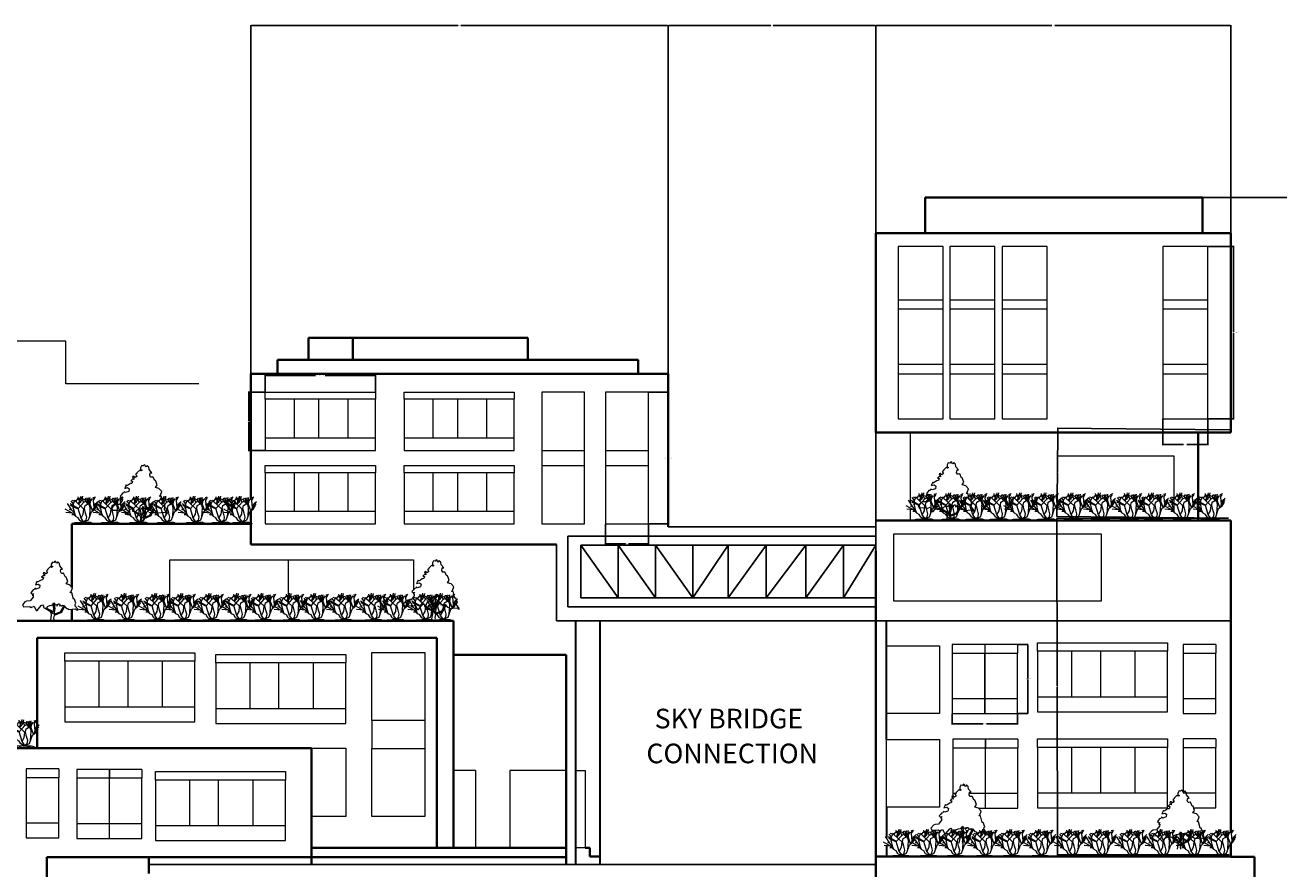
# Model space of a CAD drawing. Units: inches. Extents: x -934 to 898, y -1502 to 444.
# Tile 9 of 10: x -117 to 286, y -87 to 185. Entities that reach past the tile are written whole.
import ezdxf

# ---------------------------------------------------------------- set-up
doc = ezdxf.new("R2010")
doc.units = ezdxf.units.IN
doc.header["$MEASUREMENT"] = 0
for name, color, linetype, lineweight in [('A-ANNO-DIMS', 2, 'Continuous', 18), ('A-ANNO-TEXT', 7, 'Continuous', 18), ('A-COLS', 1, 'Continuous', 30), ('A-ELEV', 7, 'Continuous', 35), ('A-GLAZ', 4, 'Continuous', 13), ('A-ROOF', 7, 'Continuous', 35), ('L-PLNT-TREE', 3, 'Continuous', 13), ('S-BRDG', 5, 'Continuous', 25)]:
    doc.layers.add(name, color=color, linetype=linetype, lineweight=lineweight)
doc.styles.get("Standard").update_dxf_attribs({"font": 'arial.ttf'})
doc.dimstyles.get("Standard").update_dxf_attribs({"dimtxt": 0.18, "dimasz": 0.18, "dimexe": 0.18, "dimexo": 0.0625, "dimgap": 0.09, "dimtad": 0, "dimtih": 1, "dimtoh": 1, "dimdec": 4, "dimzin": 0, "dimdsep": 46, "dimtxsty": 'Standard', "dimcen": 0.09, "dimadec": 0, "dimazin": 0, "dimtfac": 1, "dimtdec": 4, "dimtofl": 0, "dimtmove": 0, "dimatfit": 3, "dimfxl": 1, "dimtolj": 1, "dimtzin": 0, "dimarcsym": 0})

# ---------------------------------------------------------------- blocks, each defined once
blk = doc.blocks.new('*U2')
for points in [[(22.0124, 137.721), (18.5475, 141.5624), (15.5282, 138.2446), (13.8028, 139.3505), (13.3714, 142.1153), (11.2148, 143.2214), (8.1954, 140.4564), (4.7447, 141.0094), (2.1567, 136.0326), (2.1567, 131.6088), (5.6074, 129.9499), (3.0193, 128.2909), (0.4313, 130.5029), (-6.9015, 123.3141), (-6.9015, 121.6552), (-9.9208, 119.9963), (-9.0581, 118.3373), (-6.9015, 115.0195), (-10.7835, 112.2546), (-14.6656, 115.0195), (-16.8222, 114.4665), (-17.6849, 112.2546), (-14.6656, 111.7016), (-14.2342, 107.2778), (-17.6065, 107.8307), (-21.5669, 103.9599), (-17.2536, 103.4069), (-18.9789, 97.8771), (-22.8609, 97.3241), (-27.1743, 94.5593), (-32.3504, 91.7944), (-32.7817, 94.0063), (-36.6638, 85.7116), (-29.7624, 87.3705), (-25.449, 84.6056), (-26.743, 77.9699), (-34.507, 75.205), (-37.9578, 77.4169), (-39.2518, 74.099), (-42.2711, 73.5461), (-44.8592, 70.2282), (-47.8786, 66.3574), (-43.9965, 63.0395), (-41.4085, 64.6985), (-44.3346, 59.8898), (-42.2089, 60.1377), (-42.5159, 55.7849), (-49.6039, 46.4502), (-58.2307, 45.8972), (-62.1127, 43.6853), (-68.5828, 36.4966), (-65.9947, 32.0727), (-50.0352, 32.6257), (-47.0159, 30.4138), (-39.6831, 33.7317), (-34.507, 22.6721), (-32.3504, 22.6721), (-22.4296, 34.8376), (-19.4102, 36.4966), (-17.2536, 33.7317), (-17.2536, 29.8608), (-13.8028, 28.7549), (-9.0581, 28.7549), (-7.3328, 32.6257), (-1.7254, 35.3906), (3.8821, 35.9436), (6.4701, 38.1555), (6.9014, 38.7085), (8.1954, 41.4734), (9.9208, 40.3674), (11.2148, 35.9436), (14.2341, 37.6025), (15.0968, 36.4966), (15.9595, 33.7317), (18.9789, 38.7085), (21.9982, 38.7085), (23.2922, 36.4966), (21.9982, 34.2847), (25.4489, 35.3906), (26.743, 33.7317), (29.7623, 35.9436), (32.7817, 34.8376), (38.8204, 28.7549), (41.4084, 27.6489), (43.5651, 25.437), (61.6813, 27.0959), (65.132, 23.7781), (67.7201, 24.884), (60.8186, 33.7317), (60.3873, 37.0495), (62.544, 40.3674), (58.662, 50.874), (56.5053, 50.874), (52.1919, 66.3574), (47.8785, 66.9103), (50.4665, 69.1222), (53.9172, 77.9699), (47.0158, 85.1586), (38.3891, 87.9235), (42.2711, 94.0063)], [(42.2711, 94.0063), (38.8204, 104.5129), (36.6637, 104.5129), (32.3503, 113.9135), (29.7623, 113.3605), (26.743, 113.3605), (24.5862, 117.7844), (25.8802, 123.8671), (29.331, 123.8671), (22.8609, 131.6088), (21.9982, 137.6916)], [(-9.9208, 28.2019), (0, 23.2251), (3.4507, 19.9072), (4.7447, 15.4834), (8.6267, 27.0959), (6.4701, 37.6025)], [(34.5071, 33.1787), (27.1743, 18.2483), (9.0581, 10.5066), (7.7641, 3.8708), (8.1954, 0)], [(8.1954, 40.3674), (11.2148, 27.6489), (8.1954, 13.8245), (24.5862, 19.9072), (32.7817, 34.2847)], [(-12.9401, 28.7549), (-2.588, 22.1191), (0.8626, 17.6953), (1.7253, 11.6125), (0, 0)]]:
    blk.add_lwpolyline(points)
blk = doc.blocks.new('*U6')
for p, q in [((-316.7634, 502.285), (-327.6092, 559.9176)), ((-286.512, 498.3226), (-307.4416, 538.0736)), ((-290.3982, 464.5406), (-265.6078, 577.8246)), ((-207.264, 451.104), (-268.224, 548.64)), ((-240.792, 502.285), (-228.3968, 573.8368)), ((-182.88, 499.872), (-158.496, 536.448)), ((-129.1844, 450.6214), (-140.0302, 542.036)), ((-134.112, 487.68), (-97.536, 548.64)), ((-85.7758, 472.4908), (-73.3552, 548.005)), ((-12.9032, 555.9552), (-2.0574, 522.1732)), ((-5.1562, 486.3846), (2.5908, 542.036)), ((-0.508, 508.254), (22.7584, 536.067)), ((1.0414, 526.1356), (35.1536, 559.9176)), ((2.5908, 542.036), (21.209, 555.9552)), ((-451.104, 219.456), (-601.0402, 303.8094)), ((-463.296, 280.416), (-552.577, 423.037)), ((-463.296, 280.416), (-512.064, 292.608)), ((-329.184, 316.992), (-499.872, 414.528)), ((-353.568, 316.992), (-487.68, 377.952)), ((-426.72, 414.528), (-475.488, 475.488)), ((-402.336, 207.264), (-463.296, 280.416)), ((-377.952, 463.296), (-451.104, 487.68)), ((-426.72, 316.992), (-451.104, 329.184)), ((-426.72, 414.528), (-390.144, 499.872)), ((-426.72, 316.992), (-426.72, 414.528)), ((-402.336, 207.264), (-426.72, 316.992)), ((-377.952, 463.296), (-329.184, 524.256)), ((-207.264, 304.8), (-377.952, 463.296)), ((-329.184, 316.992), (-353.568, 316.992)), ((-338.455, 424.7896), (-290.3982, 464.5406)), ((-329.184, 316.992), (-207.264, 451.104)), ((-268.224, 109.728), (-329.184, 316.992)), ((-296.5958, 484.4034), (-316.7634, 502.285)), ((-305.8922, 396.9512), (-302.7934, 478.4344)), ((-304.3428, 426.7708), (-268.7066, 458.5716)), ((-302.7934, 478.4344), (-270.256, 518.1854)), ((-268.7066, 458.5716), (-250.0884, 500.3038)), ((-182.88, 499.872), (-219.456, 512.064)), ((-219.456, 195.072), (-207.264, 304.8)), ((-207.264, 451.104), (-134.112, 487.68)), ((-195.072, 316.992), (-182.88, 377.952)), ((-170.688, 219.456), (-195.072, 316.992)), ((-121.92, 414.528), (-182.88, 499.872)), ((-182.88, 377.952), (-97.536, 426.72)), ((-85.7758, 389.001), (-129.1844, 452.6026)), ((-73.152, 329.184), (-109.728, 499.872)), ((-97.536, 426.72), (-24.384, 524.256)), ((-70.2564, 426.7708), (-85.7758, 472.4908)), ((-85.344, 134.112), (-73.152, 329.184)), ((-73.152, 402.336), (-60.96, 512.064)), ((-24.384, 268.224), (-73.152, 402.336)), ((-48.768, 243.84), (24.384, 304.8)), ((-12.192, 274.32), (8.7884, 335.3562)), ((8.7884, 335.3562), (-5.1562, 486.3846)), ((-3.6068, 492.3536), (14.986, 518.1854)), ((8.7884, 335.3562), (33.6042, 412.8516)), ((24.384, 304.8), (36.576, 390.144)), ((24.384, 304.8), (73.152, 377.952)), ((33.6042, 412.8516), (92.5068, 464.5406)), ((36.576, 390.144), (73.152, 438.912)), ((48.768, 341.376), (60.96, 390.144)), ((60.96, 390.144), (85.344, 414.528)), ((-451.104, 219.456), (-587.4512, 234.2388)), ((-414.528, 182.88), (-463.296, 182.88)), ((-377.952, 146.304), (-451.104, 219.456)), ((-402.336, 12.192), (-451.104, 0)), ((-377.952, 146.304), (-402.336, 207.264)), ((-341.376, 12.192), (-402.336, 12.192)), ((-329.184, 121.92), (-377.952, 146.304)), ((-243.84, 24.384), (-341.376, 12.192)), ((-292.608, 60.96), (-329.184, 121.92)), ((-243.84, 24.384), (-329.184, 0)), ((-219.456, 24.384), (-292.608, 60.96)), ((-268.224, 109.728), (-219.456, 195.072)), ((-219.456, 48.768), (-268.224, 109.728)), ((-243.84, 24.384), (-195.072, 24.384)), ((-219.456, 24.384), (-109.728, 73.152)), ((-219.456, 24.384), (-158.496, 73.152)), ((-219.456, 24.384), (-219.456, 48.768)), ((-219.456, 24.384), (-73.152, 24.384)), ((-195.072, 24.384), (-158.496, 12.192)), ((-146.304, 134.112), (-170.688, 219.456)), ((-158.496, 73.152), (-146.304, 134.112)), ((-158.496, 12.192), (-85.344, 0)), ((-109.728, 73.152), (-48.768, 243.84)), ((-73.152, 24.384), (0, 0))]:
    blk.add_line(p, q)
blk = doc.blocks.new('*U4')
for points in [[(559.11496, 3498.1134), (471.1065, 3595.68496), (394.41628, 3511.41284), (350.59112, 3539.5027), (339.63356, 3609.72862), (284.85592, 3637.82356), (208.16316, 3567.59256), (120.51538, 3581.63876), (54.78018, 3455.22804), (54.78018, 3342.86352), (142.42796, 3300.72746), (76.69022, 3258.58886), (10.95502, 3314.77366), (-175.2981, 3132.17814), (-175.2981, 3090.04208), (-251.98832, 3047.90602), (-230.07574, 3005.76742), (-175.2981, 2921.4953), (-273.9009, 2851.26684), (-372.50624, 2921.4953), (-427.28388, 2907.4491), (-449.19646, 2851.26684), (-372.50624, 2837.22064), (-361.54868, 2724.85612), (-447.2051, 2738.89978), (-547.79926, 2640.58146), (-438.24144, 2626.53526), (-482.06406, 2486.07834), (-580.66686, 2472.03214), (-690.22722, 2401.80622), (-821.70016, 2331.57776), (-832.65518, 2387.76002), (-931.26052, 2177.07464), (-755.96496, 2219.2107), (-646.4046, 2148.98224), (-679.2722, 1980.43546), (-876.4778, 1910.207), (-964.12812, 1966.38926), (-996.99572, 1882.1146), (-1073.68594, 1868.07094), (-1139.42368, 1783.79628), (-1216.11644, 1685.47796), (-1117.5111, 1601.2033), (-1051.7759, 1643.3419), (-1126.09884, 1521.20092), (-1072.10606, 1527.49758), (-1079.90386, 1416.93646), (-1259.93906, 1179.83508), (-1479.05978, 1165.78888), (-1577.66258, 1109.60662), (-1742.00312, 927.01364), (-1676.26538, 814.64658), (-1270.89408, 828.69278), (-1194.20386, 772.51052), (-1007.95074, 856.78518), (-876.4778, 575.87134), (-821.70016, 575.87134), (-569.71184, 884.87504), (-493.01908, 927.01364), (-438.24144, 856.78518), (-438.24144, 758.46432), (-350.59112, 730.37446), (-230.07574, 730.37446), (-186.25312, 828.69278), (-43.82516, 898.92124), (98.60534, 912.96744), (164.34054, 969.1497), (175.29556, 983.1959), (208.16316, 1053.42436), (251.98832, 1025.33196), (284.85592, 912.96744), (361.54614, 955.1035), (383.45872, 927.01364), (405.3713, 856.78518), (482.06406, 983.1959), (558.75428, 983.1959), (591.62188, 927.01364), (558.75428, 870.83138), (646.40206, 898.92124), (679.2722, 856.78518), (755.96242, 912.96744), (832.65518, 884.87504), (986.03816, 730.37446), (1051.77336, 702.28206), (1106.55354, 646.0998), (1566.70502, 688.23586), (1654.3528, 603.96374), (1720.09054, 632.0536), (1544.79244, 856.78518), (1533.83742, 941.0573), (1588.6176, 1025.33196), (1490.0148, 1292.1996), (1435.23462, 1292.1996), (1325.67426, 1685.47796), (1216.1139, 1699.52162), (1281.8491, 1755.70388), (1369.49688, 1980.43546), (1194.20132, 2163.02844), (975.08314, 2233.2569), (1073.68594, 2387.76002)], [(1073.68594, 2387.76002), (986.03816, 2654.62766), (931.25798, 2654.62766), (821.69762, 2893.4029), (755.96242, 2879.3567), (679.2722, 2879.3567), (624.48948, 2991.72376), (657.35708, 3146.22434), (745.0074, 3146.22434), (580.66686, 3342.86352), (558.75428, 3497.36664)], [(-251.98832, 716.32826), (0, 589.91754), (87.64778, 505.64288), (120.51538, 393.27836), (219.11818, 688.23586), (164.34054, 955.1035)], [(876.48034, 842.73898), (690.22722, 463.50682), (230.07574, 266.86764), (197.20814, 98.31832), (208.16316, 0)], [(208.16316, 1025.33196), (284.85592, 702.28206), (208.16316, 351.1423), (624.48948, 505.64288), (832.65518, 870.83138)], [(-328.67854, 730.37446), (-65.7352, 561.82514), (21.91004, 449.46062), (43.82262, 294.9575), (0, 0)]]:
    blk.add_lwpolyline(points)
blk = doc.blocks.new('WIN-TWIN-NARROW')
for p, q in [((10.5, 22.21), (0, 22.21)), ((0, 22.21), (0, 19.45)), ((20.91, 22.21), (10.41, 22.21)), ((10.41, 22.21), (10.41, 19.45)), ((10.5, 22.21), (10.5, 19.45)), ((20.91, 22.21), (20.91, 19.45)), ((0, 19.45), (0, 4.84)), ((0, 19.45), (10.5, 19.45)), ((10.41, 19.45), (10.41, 4.84)), ((10.41, 19.45), (20.91, 19.45)), ((10.5, 4.84), (10.5, 19.45)), ((20.91, 4.84), (20.91, 19.45)), ((0, 4.84), (10.5, 4.84)), ((0, 4.84), (0, 0)), ((10.41, 4.84), (20.91, 4.84)), ((10.41, 4.84), (10.41, 0)), ((10.5, 0), (10.5, 4.84)), ((20.91, 0), (20.91, 4.84)), ((0, 0), (10.5, 0)), ((10.41, 0), (20.91, 0))]:
    blk.add_line(p, q)
blk = doc.blocks.new('WIN-SINGLE-NARROW')
for p, q in [((10.5, 22.21), (0, 22.21)), ((0, 22.21), (0, 19.45)), ((10.5, 22.21), (10.5, 19.45)), ((0, 19.45), (0, 4.84)), ((0, 19.45), (10.5, 19.45)), ((10.5, 4.84), (10.5, 19.45)), ((0, 4.84), (10.5, 4.84)), ((0, 4.84), (0, 0)), ((10.5, 0), (10.5, 4.84)), ((0, 0), (10.5, 0))]:
    blk.add_line(p, q)
blk = doc.blocks.new('WIN-RIBBON-LARGE')
for p, q in [((0, 19.45), (0, 22.21)), ((0, 22.21), (41.85, 22.21)), ((41.85, 22.21), (41.85, 19.45)), ((0, 19.45), (0, 4.84)), ((41.85, 19.45), (0, 19.45)), ((10.96, 19.45), (10.96, 4.84)), ((20.23, 19.45), (20.23, 4.84)), ((31.34, 19.45), (31.34, 4.84)), ((41.85, 4.84), (41.85, 19.45)), ((0, 4.84), (41.85, 4.84)), ((0, 4.84), (0, 0)), ((41.85, 0), (41.85, 4.84)), ((0, 0), (41.85, 0))]:
    blk.add_line(p, q)
blk = doc.blocks.new('WIN-RIBBON-COMPACT')
for p, q in [((0, 16.47), (0, 18.8)), ((0, 18.8), (35.42, 18.8)), ((0, 16.47), (0, 4.09)), ((35.42, 16.47), (0, 16.47)), ((9.28, 16.47), (9.28, 4.09)), ((17.13, 16.47), (17.13, 4.09)), ((26.53, 16.47), (26.53, 4.09)), ((35.42, 18.8), (35.42, 16.47)), ((35.42, 4.09), (35.42, 16.47)), ((0, 4.09), (35.42, 4.09)), ((0, 4.09), (0, 0)), ((35.42, 0), (35.42, 4.09)), ((0, 0), (35.42, 0))]:
    blk.add_line(p, q)
blk = doc.blocks.new('WIN-TOWER-STACK')
for p, q in [((0, 55.38), (0, 0)), ((14.46, 55.38), (0, 55.38)), ((14.46, 0), (14.46, 55.38)), ((0, 38.19), (14.46, 38.19)), ((0, 35.32), (14.46, 35.32)), ((0, 17.59), (14.46, 17.59)), ((0, 14.39), (14.46, 14.39)), ((0, 0), (14.46, 0))]:
    blk.add_line(p, q)
blk = doc.blocks.new('WIN-VERTICAL-LIGHT')
for p, q in [((0, 42.42), (0, 0)), ((13.76, 42.42), (0, 42.42)), ((13.76, 0), (13.76, 42.42)), ((0, 23.62), (13.76, 23.62)), ((0, 18.8), (13.76, 18.8)), ((0, 0), (13.76, 0))]:
    blk.add_line(p, q)
blk = doc.blocks.new('*D35')
at = {"layer": 'A-ANNO-DIMS', "color": 0, "lineweight": -2, "transparency": 16777216}
for p, q in [((202.02, -14.7), (205.47, -14.7)), ((205.29, -14.88), (205.29, -25.62)), ((205.29, -36.73), (205.29, -25.99)), ((202.02, -36.91), (205.47, -36.91))]:
    blk.add_line(p, q, dxfattribs=at)
at = {"layer": 'A-ANNO-DIMS', "color": 0, "transparency": 16777216}
for points in [[(205.26, -14.88), (205.32, -14.88), (205.29, -14.7)], [(205.26, -36.73), (205.32, -36.73), (205.29, -36.91)]]:
    blk.add_solid(points, dxfattribs=at)
at = {"layer": 'Defpoints', "color": 0, "transparency": 16777216}
for p in [(201.96, -14.7), (205.29, -14.7), (201.96, -36.91)]:
    blk.add_point(p, dxfattribs=at)
at = {"layer": 'A-ANNO-DIMS', "color": 0, "transparency": 16777216, "insert": (205.29, -25.8), "char_height": 0.18, "attachment_point": 5}
blk.add_mtext('\\A1;SLIM TWIN 22 TYP.', dxfattribs=at)
blk = doc.blocks.new('*D36')
at = {"layer": 'A-ANNO-DIMS', "color": 0, "lineweight": -2, "transparency": 16777216}
for p, q in [((181.05, -36.97), (181.05, -40.42)), ((181.23, -40.24), (190.98, -40.24)), ((201.78, -40.24), (192.04, -40.24)), ((201.96, -36.97), (201.96, -40.42))]:
    blk.add_line(p, q, dxfattribs=at)
at = {"layer": 'A-ANNO-DIMS', "color": 0, "transparency": 16777216}
for points in [[(181.23, -40.21), (181.23, -40.27), (181.05, -40.24)], [(201.78, -40.21), (201.78, -40.27), (201.96, -40.24)]]:
    blk.add_solid(points, dxfattribs=at)
at = {"layer": 'Defpoints', "color": 0, "transparency": 16777216}
for p in [(181.05, -36.91), (201.96, -36.91), (201.96, -40.24)]:
    blk.add_point(p, dxfattribs=at)
at = {"layer": 'A-ANNO-DIMS', "color": 0, "transparency": 16777216, "insert": (191.51, -40.24), "char_height": 0.18, "attachment_point": 5}
blk.add_mtext('\\A1;21 TYP.', dxfattribs=at)
blk = doc.blocks.new('*D41')
at = {"layer": 'A-ANNO-DIMS', "color": 0, "lineweight": -2, "transparency": 16777216}
for p, q in [((-39.96, 66.58), (-39.96, 72.01)), ((-39.78, 71.83), (-23.77, 71.83)), ((-4.72, 71.83), (-20.73, 71.83)), ((-4.54, 66.58), (-4.54, 72.01))]:
    blk.add_line(p, q, dxfattribs=at)
at = {"layer": 'A-ANNO-DIMS', "color": 0, "transparency": 16777216}
for points in [[(-39.78, 71.86), (-39.78, 71.8), (-39.96, 71.83)], [(-4.72, 71.86), (-4.72, 71.8), (-4.54, 71.83)]]:
    blk.add_solid(points, dxfattribs=at)
at = {"layer": 'Defpoints', "color": 0, "transparency": 16777216}
for p in [(-4.54, 71.83), (-39.96, 66.52), (-4.54, 66.52)]:
    blk.add_point(p, dxfattribs=at)
at = {"layer": 'A-ANNO-DIMS', "color": 0, "transparency": 16777216, "insert": (-22.25, 71.83), "char_height": 0.18, "attachment_point": 5}
blk.add_mtext('\\A1;SHORT RIBBON 35 TYP.', dxfattribs=at)
blk = doc.blocks.new('*D42')
at = {"layer": 'A-ANNO-DIMS', "color": 0, "lineweight": -2, "transparency": 16777216}
for p, q in [((-40.03, 66.52), (-45.46, 66.52)), ((-45.28, 66.34), (-45.28, 57.3)), ((-45.28, 47.9), (-45.28, 56.94)), ((-40.03, 47.72), (-45.46, 47.72))]:
    blk.add_line(p, q, dxfattribs=at)
at = {"layer": 'A-ANNO-DIMS', "color": 0, "transparency": 16777216}
for points in [[(-45.31, 66.34), (-45.25, 66.34), (-45.28, 66.52)], [(-45.31, 47.9), (-45.25, 47.9), (-45.28, 47.72)]]:
    blk.add_solid(points, dxfattribs=at)
at = {"layer": 'Defpoints', "color": 0, "transparency": 16777216}
for p in [(-45.28, 66.52), (-39.96, 66.52), (-39.96, 47.72)]:
    blk.add_point(p, dxfattribs=at)
at = {"layer": 'A-ANNO-DIMS', "color": 0, "transparency": 16777216, "insert": (-45.28, 57.12), "char_height": 0.18, "attachment_point": 5}
blk.add_mtext('\\A1;19 TYP.', dxfattribs=at)
blk = doc.blocks.new('*D43')
at = {"layer": 'A-ANNO-DIMS', "color": 0, "lineweight": -2, "transparency": 16777216}
for p, q in [((263.27, 113.31), (271.69, 113.31)), ((271.51, 113.13), (271.51, 85.81)), ((271.51, 58.11), (271.51, 85.44)), ((263.27, 57.93), (271.69, 57.93))]:
    blk.add_line(p, q, dxfattribs=at)
at = {"layer": 'A-ANNO-DIMS', "color": 0, "transparency": 16777216}
for points in [[(271.48, 113.13), (271.54, 113.13), (271.51, 113.31)], [(271.48, 58.11), (271.54, 58.11), (271.51, 57.93)]]:
    blk.add_solid(points, dxfattribs=at)
at = {"layer": 'Defpoints', "color": 0, "transparency": 16777216}
for p in [(263.21, 113.31), (271.51, 113.31), (263.21, 57.93)]:
    blk.add_point(p, dxfattribs=at)
at = {"layer": 'A-ANNO-DIMS', "color": 0, "transparency": 16777216, "insert": (271.51, 85.62), "char_height": 0.18, "attachment_point": 5}
blk.add_mtext('\\A1;TOWER LIGHT 55 TYP.', dxfattribs=at)
blk = doc.blocks.new('*D44')
at = {"layer": 'A-ANNO-DIMS', "color": 0, "lineweight": -2, "transparency": 16777216}
for p, q in [((248.75, 57.87), (248.75, 49.45)), ((263.21, 57.87), (263.21, 49.45)), ((248.93, 49.63), (255.46, 49.63)), ((263.03, 49.63), (256.5, 49.63))]:
    blk.add_line(p, q, dxfattribs=at)
at = {"layer": 'A-ANNO-DIMS', "color": 0, "transparency": 16777216}
for points in [[(248.93, 49.66), (248.93, 49.6), (248.75, 49.63)], [(263.03, 49.66), (263.03, 49.6), (263.21, 49.63)]]:
    blk.add_solid(points, dxfattribs=at)
at = {"layer": 'Defpoints', "color": 0, "transparency": 16777216}
for p in [(248.75, 57.93), (263.21, 57.93), (263.21, 49.63)]:
    blk.add_point(p, dxfattribs=at)
at = {"layer": 'A-ANNO-DIMS', "color": 0, "transparency": 16777216, "insert": (255.98, 49.63), "char_height": 0.18, "attachment_point": 5}
blk.add_mtext('\\A1;14 TYP.', dxfattribs=at)
blk = doc.blocks.new('*D45')
at = {"layer": 'A-ANNO-DIMS', "color": 0, "lineweight": -2, "transparency": 16777216}
for p, q in [((83.35, 66.52), (89.83, 66.52)), ((89.65, 66.34), (89.65, 45.49)), ((89.65, 24.28), (89.65, 45.12)), ((83.35, 24.1), (89.83, 24.1))]:
    blk.add_line(p, q, dxfattribs=at)
at = {"layer": 'A-ANNO-DIMS', "color": 0, "transparency": 16777216}
for points in [[(89.62, 66.34), (89.68, 66.34), (89.65, 66.52)], [(89.62, 24.28), (89.68, 24.28), (89.65, 24.1)]]:
    blk.add_solid(points, dxfattribs=at)
at = {"layer": 'Defpoints', "color": 0, "transparency": 16777216}
for p in [(83.29, 66.52), (89.65, 66.52), (83.29, 24.1)]:
    blk.add_point(p, dxfattribs=at)
at = {"layer": 'A-ANNO-DIMS', "color": 0, "transparency": 16777216, "insert": (89.65, 45.31), "char_height": 0.18, "attachment_point": 5}
blk.add_mtext('\\A1;VERT. LIGHT 42 TYP.', dxfattribs=at)
blk = doc.blocks.new('*D46')
at = {"layer": 'A-ANNO-DIMS', "color": 0, "lineweight": -2, "transparency": 16777216}
for p, q in [((69.53, 24.03), (69.53, 17.55)), ((83.29, 24.03), (83.29, 17.55)), ((69.71, 17.73), (75.89, 17.73)), ((83.11, 17.73), (76.93, 17.73))]:
    blk.add_line(p, q, dxfattribs=at)
at = {"layer": 'A-ANNO-DIMS', "color": 0, "transparency": 16777216}
for points in [[(69.71, 17.76), (69.71, 17.7), (69.53, 17.73)], [(83.11, 17.76), (83.11, 17.7), (83.29, 17.73)]]:
    blk.add_solid(points, dxfattribs=at)
at = {"layer": 'Defpoints', "color": 0, "transparency": 16777216}
for p in [(69.53, 24.1), (83.29, 24.1), (83.29, 17.73)]:
    blk.add_point(p, dxfattribs=at)
at = {"layer": 'A-ANNO-DIMS', "color": 0, "transparency": 16777216, "insert": (76.41, 17.73), "char_height": 0.18, "attachment_point": 5}
blk.add_mtext('\\A1;14 TYP.', dxfattribs=at)
blk = doc.blocks.new('*D80')
at = {"layer": 'A-ANNO-DIMS', "color": 0, "lineweight": -2, "transparency": 16777216}
for p, q in [((261.62, 129.1), (464.31, 129.1)), ((464.13, 128.92), (464.13, -24.61)), ((464.13, -178.5), (464.13, -24.97)), ((239.7, -178.68), (464.31, -178.68))]:
    blk.add_line(p, q, dxfattribs=at)
at = {"layer": 'A-ANNO-DIMS', "color": 0, "transparency": 16777216}
for points in [[(464.1, 128.92), (464.16, 128.92), (464.13, 129.1)], [(464.1, -178.5), (464.16, -178.5), (464.13, -178.68)]]:
    blk.add_solid(points, dxfattribs=at)
at = {"layer": 'Defpoints', "color": 0, "transparency": 16777216}
for p in [(261.56, 129.1), (464.13, 129.1), (239.64, -178.68)]:
    blk.add_point(p, dxfattribs=at)
at = {"layer": 'A-ANNO-DIMS', "color": 0, "transparency": 16777216, "insert": (464.13, -24.79), "char_height": 0.18, "attachment_point": 5}
blk.add_mtext('\\A1;307.8', dxfattribs=at)
blk = doc.blocks.new('*D83')
at = {"layer": 'A-ANNO-DIMS', "color": 0, "lineweight": -2, "transparency": 16777216}
for p, q in [((156.42, 117.65), (156.42, 184.53)), ((156.6, 184.35), (213.08, 184.35)), ((270.46, 184.35), (213.99, 184.35)), ((270.64, 117.65), (270.64, 184.53))]:
    blk.add_line(p, q, dxfattribs=at)
at = {"layer": 'A-ANNO-DIMS', "color": 0, "transparency": 16777216}
for points in [[(156.6, 184.38), (156.6, 184.32), (156.42, 184.35)], [(270.46, 184.38), (270.46, 184.32), (270.64, 184.35)]]:
    blk.add_solid(points, dxfattribs=at)
at = {"layer": 'Defpoints', "color": 0, "transparency": 16777216}
for p in [(270.64, 184.35), (156.42, 117.59), (270.64, 117.59)]:
    blk.add_point(p, dxfattribs=at)
at = {"layer": 'A-ANNO-DIMS', "color": 0, "transparency": 16777216, "insert": (213.53, 184.35), "char_height": 0.18, "attachment_point": 5}
blk.add_mtext('\\A1;114.22', dxfattribs=at)
blk = doc.blocks.new('*D86')
at = {"layer": 'A-ANNO-DIMS', "color": 0, "lineweight": -2, "transparency": 16777216}
for p, q in [((-44.58, 72.4), (-44.58, 184.53)), ((-44.4, 184.35), (22.08, 184.35)), ((89.46, 184.35), (22.98, 184.35)), ((89.64, 72.4), (89.64, 184.53))]:
    blk.add_line(p, q, dxfattribs=at)
at = {"layer": 'A-ANNO-DIMS', "color": 0, "transparency": 16777216}
for points in [[(-44.4, 184.38), (-44.4, 184.32), (-44.58, 184.35)], [(89.46, 184.38), (89.46, 184.32), (89.64, 184.35)]]:
    blk.add_solid(points, dxfattribs=at)
at = {"layer": 'Defpoints', "color": 0, "transparency": 16777216}
for p in [(89.64, 184.35), (-44.58, 72.34), (89.64, 72.34)]:
    blk.add_point(p, dxfattribs=at)
at = {"layer": 'A-ANNO-DIMS', "color": 0, "transparency": 16777216, "insert": (22.53, 184.35), "char_height": 0.18, "attachment_point": 5}
blk.add_mtext('\\A1;134.22', dxfattribs=at)
blk = doc.blocks.new('*D87')
at = {"layer": 'A-ANNO-DIMS', "color": 0, "lineweight": -2, "transparency": 16777216}
for p, q in [((89.64, 23.19), (89.64, 184.53)), ((89.82, 184.35), (122.64, 184.35)), ((156.24, 184.35), (123.43, 184.35)), ((156.42, 23.19), (156.42, 184.53))]:
    blk.add_line(p, q, dxfattribs=at)
at = {"layer": 'A-ANNO-DIMS', "color": 0, "transparency": 16777216}
for points in [[(89.82, 184.38), (89.82, 184.32), (89.64, 184.35)], [(156.24, 184.38), (156.24, 184.32), (156.42, 184.35)]]:
    blk.add_solid(points, dxfattribs=at)
at = {"layer": 'Defpoints', "color": 0, "transparency": 16777216}
for p in [(156.42, 184.35), (89.64, 23.13), (156.42, 23.13)]:
    blk.add_point(p, dxfattribs=at)
at = {"layer": 'A-ANNO-DIMS', "color": 0, "transparency": 16777216, "insert": (123.03, 184.35), "char_height": 0.18, "attachment_point": 5}
blk.add_mtext('\\A1;66.78', dxfattribs=at)
blk = doc.blocks.new('*D89')
at = {"layer": 'A-ANNO-DIMS', "color": 0, "lineweight": -2, "transparency": 16777216}
for p, q in [((270.16, 54.39), (214.8, 54.91)), ((214.98, 54.73), (214.85, 40.87)), ((214.71, 26.64), (214.84, 40.5)), ((269.89, 25.94), (214.53, 26.46))]:
    blk.add_line(p, q, dxfattribs=at)
at = {"layer": 'A-ANNO-DIMS', "color": 0, "transparency": 16777216}
for points in [[(214.95, 54.73), (215.01, 54.73), (214.98, 54.91)], [(214.68, 26.64), (214.74, 26.64), (214.71, 26.46)]]:
    blk.add_solid(points, dxfattribs=at)
at = {"layer": 'Defpoints', "color": 0, "transparency": 16777216}
for p in [(214.98, 54.91), (270.23, 54.39), (269.96, 25.94)]:
    blk.add_point(p, dxfattribs=at)
at = {"layer": 'A-ANNO-DIMS', "color": 0, "transparency": 16777216, "insert": (214.84, 40.69), "char_height": 0.18, "attachment_point": 5}
blk.add_mtext('\\A1;28.45', dxfattribs=at)
blk = doc.blocks.new('*D90')
at = {"layer": 'A-ANNO-DIMS', "color": 0, "lineweight": -2, "transparency": 16777216}
for p, q in [((269.89, 25.94), (214.53, 25.86)), ((214.71, 25.68), (214.78, -28.06)), ((214.86, -82.15), (214.78, -28.42)), ((270.05, -82.26), (214.68, -82.33))]:
    blk.add_line(p, q, dxfattribs=at)
at = {"layer": 'A-ANNO-DIMS', "color": 0, "transparency": 16777216}
for points in [[(214.74, 25.68), (214.68, 25.68), (214.71, 25.86)], [(214.89, -82.15), (214.83, -82.15), (214.86, -82.33)]]:
    blk.add_solid(points, dxfattribs=at)
at = {"layer": 'Defpoints', "color": 0, "transparency": 16777216}
for p in [(214.71, 25.86), (269.96, 25.94), (270.11, -82.26)]:
    blk.add_point(p, dxfattribs=at)
at = {"layer": 'A-ANNO-DIMS', "color": 0, "transparency": 16777216, "insert": (214.78, -28.24), "char_height": 0.18, "attachment_point": 5}
blk.add_mtext('\\A1;108.2', dxfattribs=at)

msp = doc.modelspace()

# ---------------------------------------------------------------- linework, layer by layer
at = {"layer": 'A-ANNO-TEXT'}
for p, q in [((-104.1148, 82.8773), (-138.836, 82.8773)), ((-104.1148, 69.1437), (-104.1148, 82.8773)), ((-61.3585, 69.1437), (-104.1148, 69.1437))]:
    msp.add_line(p, q, dxfattribs=at)
at = {"layer": 'A-COLS'}
for p, q in [((59.8691, -7.0768), (59.8691, -85.4234)), ((67.6239, -7.0768), (67.6239, -85.4234)), ((159.8346, -45.2684), (159.8346, -7.0768)), ((159.8346, -67.0531), (159.8346, -76.8096)), ((159.8346, -79.401), (159.8346, -82.9144))]:
    msp.add_line(p, q, dxfattribs=at)
at = {"layer": 'A-ELEV'}
for p, q in [((156.4222, 117.5909), (270.6435, 117.5909)), ((156.4222, 53.4791), (156.4222, 117.5909)), ((270.6435, 95.2845), (270.6435, 117.5909)), ((270.6435, 95.2845), (270.6435, 53.4791)), ((-44.5811, 62.759), (-44.5811, 72.337)), ((-44.5811, 72.337), (85.1446, 72.337)), ((85.1446, 72.337), (89.6402, 72.337)), ((89.6402, 72.337), (89.6402, 23.1285)), ((-44.5811, 46.4182), (-44.5811, 62.759)), ((167.6187, 53.4791), (156.4222, 53.4791)), ((156.4222, 53.4791), (270.6435, 53.4791)), ((260.0938, 25.2357), (260.0938, 53.4791)), ((-44.5811, 46.4182), (-44.5811, 32.1827)), ((-44.5811, 28.4331), (-44.5811, 18.9757)), ((156.4222, 25.2357), (270.6435, 25.2357)), ((270.6435, -7.0768), (270.6435, 25.2357)), ((270.6435, 25.2357), (270.6435, 23.7503)), ((270.6435, 25.2357), (270.6435, -74.9041)), ((-44.5811, 24.0974), (-102.1424, 24.0974)), ((-102.1424, 24.0974), (-102.1424, 3.6926)), ((-44.5811, 17.5052), (-44.5811, 18.9757)), ((53.7309, 17.5052), (-44.5811, 17.5052)), ((156.4222, -7.0768), (156.4222, 15.4465)), ((-102.1424, -3.2919), (-102.1424, -7.0768)), ((20.5463, -7.0768), (-159.7746, -7.0768)), ((20.5463, -7.0768), (20.5463, -80.1164)), ((156.4222, -7.0768), (156.4222, -82.9144)), ((15.2074, -12.5592), (-113.3269, -12.5592)), ((-113.3269, -12.5592), (-113.3269, -41.0733)), ((15.2074, -12.5592), (15.2074, -80.1164)), ((20.5463, -17.9816), (56.8309, -17.9816)), ((56.8309, -17.9816), (56.8309, -85.4234)), ((-113.3269, -42.2344), (-113.3269, -47.999)), ((-113.3269, -47.999), (-397.2277, -47.999)), ((-25.055, -47.999), (-113.3269, -47.999)), ((-25.055, -80.1164), (-25.055, -47.999)), ((270.8929, -74.9041), (271.1304, -74.9041)), ((15.2074, -80.1164), (-25.055, -80.1164)), ((-25.055, -80.1164), (-25.055, -85.4234)), ((-25.055, -80.1164), (56.8309, -80.1164)), ((62.9251, -80.1164), (64.4649, -80.1164)), ((64.4649, -80.1164), (64.4649, -82.8965)), ((270.6435, -82.9144), (270.6435, -78.7963)), ((-25.055, -83.1318), (-110.2409, -83.1318)), ((-110.2409, -83.1318), (-110.2409, -85.4234)), ((-77.3547, -85.4234), (-77.3547, -83.1318)), ((-25.055, -83.1318), (56.8309, -83.1318)), ((64.4649, -82.8965), (67.6239, -82.8965)), ((156.4222, -82.9144), (270.6435, -82.9144)), ((156.4222, -82.9144), (156.4222, -122.024)), ((270.6435, -82.924), (278.229, -82.924)), ((278.229, -82.924), (278.229, -122.024)), ((-110.2409, -85.4234), (-110.2409, -151.3215)), ((-77.3547, -88.3005), (-77.3547, -85.4234))]:
    msp.add_line(p, q, dxfattribs=at)
at = {"layer": 'A-GLAZ'}
for p, q in [((167.6187, 30.7358), (167.6187, 53.4791)), ((214.8504, 46.0441), (252.2849, 46.0441)), ((214.8504, 33.6501), (214.8504, 46.0441)), ((252.2849, 46.0441), (252.2849, 27.892)), ((167.6187, 25.2357), (167.6187, 28.7475)), ((214.8504, 28.8265), (214.8504, 29.7729)), ((252.2849, 25.4938), (252.2849, 25.2357)), ((229.0594, 20.8519), (162.1205, 20.8519)), ((162.1205, 20.8519), (162.1205, -0.6479)), ((229.0594, -0.6479), (229.0594, 20.8519)), ((-70.5942, 12.564), (7.7694, 12.564)), ((-70.5942, -0.5252), (-70.5942, 12.564)), ((-32.5878, 12.564), (-32.5878, -1.6333)), ((7.7694, 12.564), (7.7694, 3.0093)), ((-70.5942, -3.5977), (-70.5942, -1.7802)), ((162.1205, -0.6479), (229.0594, -0.6479)), ((-32.5878, -6.7493), (-32.5878, -7.0768)), ((7.9526, -7.0221), (7.9526, -7.0768)), ((159.8346, -15.122), (176.9047, -15.122)), ((159.8346, -36.9067), (159.8346, -15.122)), ((176.9047, -15.122), (176.9047, -36.9067)), ((-5.6807, -17.31), (11.3893, -17.31)), ((-5.6807, -39.0947), (-5.6807, -17.31)), ((11.3893, -17.31), (11.3893, -39.0947)), ((11.3893, -39.0947), (-5.6807, -39.0947)), ((-5.6807, -39.0947), (-5.6807, -48.1857)), ((11.3893, -39.0947), (11.3893, -48.1857)), ((176.9047, -36.9067), (159.8346, -36.9067)), ((-25.055, -47.999), (-14.0528, -47.999)), ((-14.0528, -47.999), (-14.0528, -69.9704)), ((-5.6807, -48.1857), (11.3893, -48.1857)), ((-5.6807, -69.9704), (-5.6807, -48.1857)), ((11.3893, -48.1857), (11.3893, -69.9704)), ((159.8346, -45.2684), (176.9047, -45.2684)), ((159.8346, -67.0531), (159.8346, -45.2684)), ((176.9047, -45.2684), (176.9047, -67.0531)), ((191.7497, -45.1505), (181.2472, -45.1505)), ((181.2472, -45.1505), (181.2472, -47.9054)), ((181.2472, -47.9054), (181.2472, -62.5237)), ((181.2472, -47.9054), (191.7497, -47.9054)), ((202.1571, -45.1505), (191.6546, -45.1505)), ((191.6546, -45.1505), (191.6546, -47.9054)), ((191.6546, -47.9054), (191.6546, -62.5237)), ((191.6546, -47.9054), (202.1571, -47.9054)), ((191.7497, -45.1505), (191.7497, -47.9054)), ((191.7497, -62.5237), (191.7497, -47.9054)), ((202.1571, -45.1505), (202.1571, -47.9054)), ((202.1571, -62.5237), (202.1571, -47.9054)), ((265.8509, -45.0049), (255.3484, -45.0049)), ((255.3484, -45.0049), (255.3484, -47.7598)), ((255.3484, -47.7598), (255.3484, -62.3781)), ((255.3484, -47.7598), (265.8509, -47.7598)), ((265.8509, -45.0049), (265.8509, -47.7598)), ((265.8509, -62.3781), (265.8509, -47.7598)), ((27.6546, -55.2367), (20.5463, -55.2367)), ((27.6546, -55.2367), (27.6546, -80.1164)), ((56.8309, -55.2367), (38.7591, -55.2367)), ((38.7591, -55.2367), (38.7591, -80.1164)), ((59.8691, -55.2367), (62.9251, -55.2367)), ((62.9251, -55.2367), (62.9251, -80.1164)), ((181.2472, -62.5237), (182.2459, -62.5237)), ((181.2472, -62.5237), (181.2472, -64.4024)), ((186.5514, -62.5237), (191.7497, -62.5237)), ((191.6546, -62.5237), (202.1571, -62.5237)), ((191.6546, -62.5237), (191.6546, -67.3591)), ((191.7497, -67.3591), (191.7497, -62.5237)), ((202.1571, -67.3591), (202.1571, -62.5237)), ((255.3484, -62.3781), (265.8509, -62.3781)), ((265.8509, -67.2135), (265.8509, -62.3781)), ((176.9047, -67.0531), (159.8346, -67.0531)), ((189.4336, -67.3591), (191.7497, -67.3591)), ((191.6546, -67.3591), (202.1571, -67.3591)), ((258.6649, -67.2135), (265.8509, -67.2135)), ((-14.0528, -69.9704), (-25.055, -69.9704)), ((11.3893, -69.9704), (-5.6807, -69.9704)), ((62.9251, -80.1164), (59.8691, -80.1164))]:
    msp.add_line(p, q, dxfattribs=at)
at = {"layer": 'A-ROOF'}
for p, q in [((172.3459, 117.5909), (172.3459, 129.1024)), ((172.3459, 129.1024), (261.5611, 129.1024)), ((261.5611, 129.1024), (261.5611, 117.5909)), ((-26.0748, 81.8985), (-26.0748, 83.9545)), ((-26.0748, 83.9545), (44.5032, 83.9545)), ((-26.0748, 76.834), (-26.0748, 81.8985)), ((-11.7526, 76.834), (-11.7526, 83.9545)), ((44.5032, 83.9545), (44.5032, 76.834)), ((-36.019, 72.337), (-36.019, 76.834)), ((-36.019, 76.834), (80.0513, 76.834)), ((80.0513, 76.834), (80.0513, 72.337))]:
    msp.add_line(p, q, dxfattribs=at)
at = {"layer": 'S-BRDG'}
for p, q in [((156.4222, 25.2357), (156.4222, 15.4465)), ((156.4222, 20.1786), (57.3889, 20.1786)), ((57.3889, -2.5438), (57.3889, 20.1786)), ((89.6402, 23.1285), (156.4222, 23.1285)), ((53.7309, 17.5052), (53.7309, -2.5438)), ((61.5891, 17.2615), (156.4222, 17.2615)), ((61.5891, 17.2615), (61.5891, 0.3133)), ((61.5891, 17.2615), (73.5895, 0.3133)), ((73.5895, 17.2615), (73.5895, 0.3133)), ((73.5895, 17.2615), (85.5397, 0.3133)), ((85.5397, 17.2615), (85.5397, 0.3133)), ((85.5397, 17.2615), (97.6094, 0.3133)), ((97.6094, 17.2615), (97.6094, 0.3133)), ((97.6094, 0.3133), (108.962, 17.2615)), ((108.962, 17.2615), (108.962, 0.3133)), ((121.1512, 17.2615), (108.962, 0.3133)), ((121.1512, 17.2615), (121.1512, 0.3133)), ((133.9379, 17.2615), (121.1512, 0.3133)), ((133.9379, 17.2615), (133.9379, 0.3133)), ((146.0075, 17.2615), (133.9379, 0.3133)), ((146.0075, 17.2615), (146.0075, 0.3133)), ((156.4222, 17.2615), (146.0075, 0.3133)), ((156.4222, -4.4188), (156.4222, 12.5294)), ((61.5891, 0.3133), (156.4222, 0.3133)), ((53.7309, -2.5438), (53.7309, -7.0768)), ((57.3889, -2.5438), (156.4222, -2.5438)), ((53.7309, -7.0768), (270.6435, -7.0768)), ((-25.055, -85.4234), (-77.3547, -85.4234)), ((-25.055, -85.4234), (59.8691, -85.4234)), ((74.4978, -85.4234), (20.5463, -85.4234)), ((74.4978, -85.4234), (156.4222, -85.4234))]:
    msp.add_line(p, q, dxfattribs=at)

# ---------------------------------------------------------------- block references
at = {"layer": 'A-GLAZ'}
for name, p in [('WIN-TOWER-STACK', (163.5915, 57.9321)), ('WIN-TOWER-STACK', (180.2252, 57.9321)), ('WIN-TOWER-STACK', (197.1147, 57.9321)), ('WIN-TOWER-STACK', (248.7485, 57.9321)), ('WIN-RIBBON-COMPACT', (-39.964, 47.718)), ('WIN-RIBBON-COMPACT', (4.7179, 47.718)), ('WIN-VERTICAL-LIGHT', (48.9816, 24.0974)), ('WIN-VERTICAL-LIGHT', (69.5303, 24.0974)), ('WIN-RIBBON-COMPACT', (-39.964, 24.0974)), ('WIN-RIBBON-COMPACT', (4.7179, 24.0974)), ('WIN-TWIN-NARROW', (181.0511, -36.9067)), ('WIN-RIBBON-LARGE', (208.4308, -36.3063)), ('WIN-SINGLE-NARROW', (255.3484, -36.9067)), ('WIN-RIBBON-LARGE', (-104.4221, -39.5378)), ('WIN-RIBBON-LARGE', (-55.8989, -40.0835)), ('WIN-RIBBON-LARGE', (208.4308, -67.2135)), ('WIN-SINGLE-NARROW', (-116.8962, -76.8685)), ('WIN-TWIN-NARROW', (-100.5977, -77.0651)), ('WIN-RIBBON-LARGE', (-75.2801, -77.7214))]:
    msp.add_blockref(name, p, dxfattribs=at)
at = {"layer": 'L-PLNT-TREE'}
for name, p, xscale, yscale, zscale in [('*U2', (-80.3333, 24.2627), 0.1315554675521508, 0.1315554675521508, 0.1315554675521508), ('*U4', (179.1266, 25.0677), 0.0052143573184964, 0.0052143573184964, 0.0052143573184964), ('*U6', (-95.1297, 24.2507), 0.0152219259934872, 0.0152219259934872, 0.0152219259934872), ('*U6', (-86.3832, 24.2507), 0.0152219259934872, 0.0152219259934872, 0.0152219259934872), ('*U6', (-77.2821, 24.2507), 0.0152219259934872, 0.0152219259934872, 0.0152219259934872), ('*U6', (-68.4175, 24.2507), 0.0152219259934872, 0.0152219259934872, 0.0152219259934872), ('*U6', (-59.0209, 24.2507), 0.0152219259934872, 0.0152219259934872, 0.0152219259934872), ('*U6', (-50.8063, 24.2507), 0.0152219259934872, 0.0152219259934872, 0.0152219259934872), ('*U6', (-44.1738, 24.2507), 0.0152219259934872, 0.0152219259934872, 0.0152219259934872), ('*U6', (175.3966, 25.3082), 0.0152219259934872, 0.0152219259934872, 0.0152219259934872), ('*U6', (184.0163, 25.3082), 0.0152219259934872, 0.0152219259934872, 0.0152219259934872), ('*U6', (191.7405, 25.3082), 0.0152219259934872, 0.0152219259934872, 0.0152219259934872), ('*U6', (199.4647, 25.3082), 0.0152219259934872, 0.0152219259934872, 0.0152219259934872), ('*U6', (206.797, 25.3082), 0.0152219259934872, 0.0152219259934872, 0.0152219259934872), ('*U6', (214.6891, 25.3082), 0.0152219259934872, 0.0152219259934872, 0.0152219259934872), ('*U6', (223.3566, 25.3082), 0.0152219259934872, 0.0152219259934872, 0.0152219259934872), ('*U6', (232.1366, 25.3082), 0.0152219259934872, 0.0152219259934872, 0.0152219259934872), ('*U6', (241.4232, 25.3082), 0.0152219259934872, 0.0152219259934872, 0.0152219259934872), ('*U6', (249.226, 25.3082), 0.0152219259934872, 0.0152219259934872, 0.0152219259934872), ('*U6', (258.3948, 25.3082), 0.0152219259934872, 0.0152219259934872, 0.0152219259934872), ('*U6', (267.4518, 25.3082), 0.0152219259934872, 0.0152219259934872, 0.0152219259934872), ('*U4', (13.5723, -6.4696), 0.0052143573184964, 0.0052143573184964, 0.0052143573184964), ('*U2', (-109.0605, -6.747), 0.1315554675521508, 0.1315554675521508, 0.1315554675521508), ('*U6', (-90.9709, -7.0221), 0.0152219259934872, 0.0152219259934872, 0.0152219259934872), ('*U6', (-81.1969, -7.0221), 0.0152219259934872, 0.0152219259934872, 0.0152219259934872), ('*U6', (-71.348, -7.0221), 0.0152219259934872, 0.0152219259934872, 0.0152219259934872), ('*U6', (-62.9545, -7.0221), 0.0152219259934872, 0.0152219259934872, 0.0152219259934872), ('*U6', (-53.9206, -7.0221), 0.0152219259934872, 0.0152219259934872, 0.0152219259934872), ('*U6', (-45.0279, -7.0221), 0.0152219259934872, 0.0152219259934872, 0.0152219259934872), ('*U6', (-37.1232, -7.0221), 0.0152219259934872, 0.0152219259934872, 0.0152219259934872), ('*U6', (-28.0893, -7.0221), 0.0152219259934872, 0.0152219259934872, 0.0152219259934872), ('*U6', (-20.1846, -7.0221), 0.0152219259934872, 0.0152219259934872, 0.0152219259934872), ('*U6', (-11.2919, -7.0221), 0.0152219259934872, 0.0152219259934872, 0.0152219259934872), ('*U6', (-1.6934, -7.0221), 0.0152219259934872, 0.0152219259934872, 0.0152219259934872), ('*U6', (5.3643, -7.0221), 0.0152219259934872, 0.0152219259934872, 0.0152219259934872), ('*U6', (14.8193, -7.0221), 0.0152219259934872, 0.0152219259934872, 0.0152219259934872), ('*U6', (20.5119, -7.0221), 0.0152219259934872, 0.0152219259934872, 0.0152219259934872), ('*U6', (-114.1107, -47.5966), 0.0152219259934872, 0.0152219259934872, 0.0152219259934872), ('*U4', (183.1895, -78.6201), 0.0052143573184964, 0.0052143573184964, 0.0052143573184964), ('*U4', (253.3329, -80.4759), 0.0052143573184964, 0.0052143573184964, 0.0052143573184964), ('*U6', (168.0176, -82.8843), 0.0152219259934872, 0.0152219259934872, 0.0152219259934872), ('*U6', (176.914, -82.8843), 0.0152219259934872, 0.0152219259934872, 0.0152219259934872), ('*U6', (185.675, -82.8843), 0.0152219259934872, 0.0152219259934872, 0.0152219259934872), ('*U6', (194.8971, -82.8843), 0.0152219259934872, 0.0152219259934872, 0.0152219259934872), ('*U6', (203.6811, -82.8843), 0.0152219259934872, 0.0152219259934872, 0.0152219259934872), ('*U6', (212.9032, -82.8843), 0.0152219259934872, 0.0152219259934872, 0.0152219259934872), ('*U6', (222.817, -82.8843), 0.0152219259934872, 0.0152219259934872, 0.0152219259934872), ('*U6', (232.4018, -82.8843), 0.0152219259934872, 0.0152219259934872, 0.0152219259934872), ('*U6', (242.2579, -82.8843), 0.0152219259934872, 0.0152219259934872, 0.0152219259934872), ('*U6', (252.0564, -82.8843), 0.0152219259934872, 0.0152219259934872, 0.0152219259934872), ('*U6', (261.9428, -82.8843), 0.0152219259934872, 0.0152219259934872, 0.0152219259934872), ('*U6', (270.9344, -82.8843), 0.0152219259934872, 0.0152219259934872, 0.0152219259934872)]:
    msp.add_blockref(name, p, dxfattribs=dict(at, xscale=xscale, yscale=yscale, zscale=zscale))

# ---------------------------------------------------------------- texts
at = {"layer": 'A-ANNO-TEXT'}
for s, p in [('SKY BRIDGE    ', (85.3101, -41.6633)), ('CONNECTION', (82.6455, -52.879))]:
    msp.add_text(s, height=6.31231, dxfattribs=at).set_placement(p)

# ---------------------------------------------------------------- dimensions: what is measured, and where the dimension line sits
at = {"layer": 'A-ANNO-DIMS'}
for base, p1, p2, picture, middle in [((89.6402, 184.3524), (-44.5811, 72.337), (89.6402, 72.337), '*D86', (22.5296, 184.3524)), ((156.4222, 184.3524), (89.6402, 23.1285), (156.4222, 23.1285), '*D87', (123.0312, 184.3524)), ((270.6435, 184.3524), (156.4222, 117.5909), (270.6435, 117.5909), '*D83', (213.5328, 184.3524))]:
    dim = msp.add_linear_dim(base=base, p1=p1, p2=p2, dimstyle='Standard', override={"dimdec": 2, "dimlfac": 1, "dimrnd": 0, "dimzin": 0, "dimdsep": 46, "dimlunit": 2}, dxfattribs=at)
    dim.commit()
    dim.dimension.update_dxf_attribs({"geometry": picture, "text_midpoint": middle})
for base, p1, p2, angle, override, picture, middle in [((464.1272, 129.1024), (239.6401, -178.6804), (261.5611, 129.1024), 90, {"dimdec": 1, "dimlfac": 1, "dimrnd": 0, "dimzin": 0, "dimdsep": 46, "dimlunit": 2}, '*D80', (464.1272, -24.789)), ((214.9792, 54.91), (269.9565, 25.9365), (270.2267, 54.3852), 89.455785, {"dimdec": 2, "dimlfac": 1, "dimrnd": 0, "dimzin": 0, "dimdsep": 46, "dimlunit": 2}, '*D89', (214.8441, 40.6856)), ((214.7065, 25.8592), (270.1077, -82.256), (269.9565, 25.9365), 90.080093, {"dimdec": 1, "dimlfac": 1, "dimrnd": 0, "dimzin": 0, "dimdsep": 46, "dimlunit": 2}, '*D90', (214.7821, -28.237))]:
    dim = msp.add_linear_dim(base=base, p1=p1, p2=p2, angle=angle, dimstyle='Standard', override=override, dxfattribs=at)
    dim.commit()
    dim.dimension.update_dxf_attribs({"geometry": picture, "text_midpoint": middle})
for base, p1, p2, text, picture, middle in [((271.5127, 113.3118), (263.2057, 57.9321), (263.2057, 113.3118), 'TOWER LIGHT <> TYP.', '*D43', (271.5127, 85.622)), ((-45.2772, 66.5165), (-39.964, 47.718), (-39.964, 66.5165), '<> TYP.', '*D42', (-45.2772, 57.1172)), ((89.6519, 66.5165), (83.289, 24.0974), (83.289, 66.5165), 'VERT. LIGHT <> TYP.', '*D45', (89.6519, 45.3069)), ((205.2924, -14.6981), (201.9611, -36.9067), (201.9611, -14.6981), 'SLIM TWIN <> TYP.', '*D35', (205.2924, -25.8024))]:
    dim = msp.add_linear_dim(base=base, p1=p1, p2=p2, angle=90, text=text, dimstyle='Standard', override={"dimdec": 0, "dimlfac": 1, "dimrnd": 0, "dimzin": 0, "dimdsep": 46, "dimlunit": 2}, dxfattribs=at)
    dim.commit()
    dim.dimension.update_dxf_attribs({"geometry": picture, "text_midpoint": middle})
for base, p1, p2, text, picture, middle in [((-4.5433, 71.8296), (-39.964, 66.5165), (-4.5433, 66.5165), 'SHORT RIBBON <> TYP.', '*D41', (-22.2536, 71.8296)), ((263.2057, 49.6252), (248.7485, 57.9321), (263.2057, 57.9321), '<> TYP.', '*D44', (255.9771, 49.6252)), ((83.289, 17.7345), (69.5303, 24.0974), (83.289, 24.0974), '<> TYP.', '*D46', (76.4096, 17.7345)), ((201.9611, -40.238), (181.0511, -36.9067), (201.9611, -36.9067), '<> TYP.', '*D36', (191.5061, -40.238))]:
    dim = msp.add_linear_dim(base=base, p1=p1, p2=p2, text=text, dimstyle='Standard', override={"dimdec": 0, "dimlfac": 1, "dimrnd": 0, "dimzin": 0, "dimdsep": 46, "dimlunit": 2}, dxfattribs=at)
    dim.commit()
    dim.dimension.update_dxf_attribs({"geometry": picture, "text_midpoint": middle})

doc.saveas('drawing.dxf')
